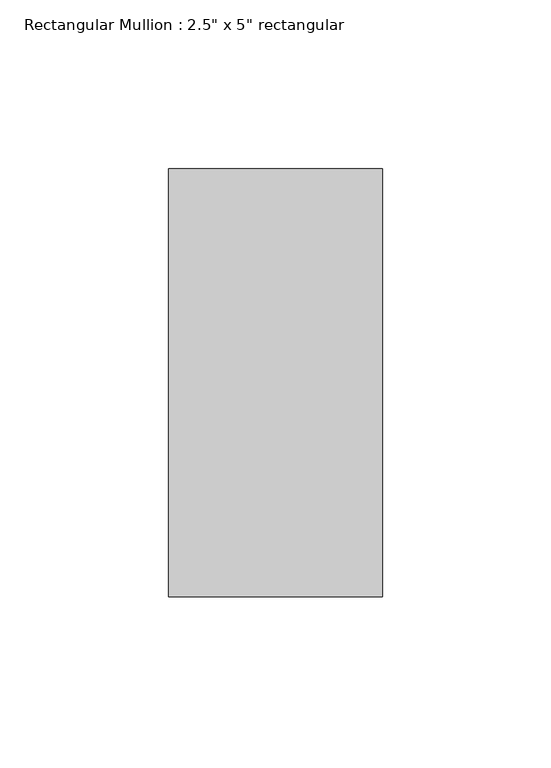
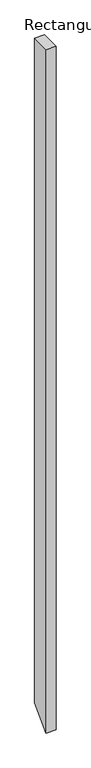
"""IFC4 building model written with IfcOpenShell, lengths in millimetres: member geometry."""

from ifc_helpers import new_model, si_unit, frame, origin, place, context, project, spatial, polyline, outline, extrude, source, transform, mapped, element, save


def member_cf286210(model_context):
    return source(origin(), model_context, "Body", "SweptSolid", [
        extrude(outline(polyline([(-63.5, 0.0), (63.5, 0.0), (63.5, -4482.350494), (-63.5, -4609.350494), (-63.5, 0.0)])), frame((-63.5, 0.0, 0.0), z_axis=(1.0, 0.0, 0.0), x_axis=(0.0, 1.0, 0.0)), (0.0, 0.0, 1.0), 63.5),
    ])


if __name__ == "__main__":
    model = new_model("IFC4")
    model_context = context("Model", 3, world=origin())
    ifc_project = project(units=[si_unit("LENGTHUNIT", "METRE", prefix="MILLI")], contexts=[model_context])
    site = spatial("IfcSite", under=ifc_project)
    building = spatial("IfcBuilding", under=site)
    placement = place(None, origin())
    member_shape = member_cf286210(model_context)
    element("IfcMember", 1, ObjectType="Rectangular Mullion : 2.5\" x 5\" rectangular", at=placement, inside=building, context=model_context, shape_type="MappedRepresentation", body=[
        mapped(member_shape, transform((0.0, 0.0, 0.0), x_axis=(1.0, 0.0, 0.0), y_axis=(0.0, 1.0, 0.0), z_axis=(0.0, 0.0, 1.0))),
    ])
    save(model, "model.ifc")

# Revit data of these elements
# Type "Rectangular Mullion : 2.5\" x 5\" rectangular"
#   built-in parameter 1007304 = 0.416667 (stored number, unit not read)
#   built-in parameter 1007301 = 0.104167 (stored number, unit not read)
#   built-in parameter 1007300 = 0.104167 (stored number, unit not read)
# Element 1 (IfcMember, "Rectangular Mullion : 2.5\" x 5\" rectangular")
#   Materials on its faces: "Aluminum"
# Materials
#   "Aluminum": class "Metal", colour RGB 247 247 247, transparency 0, Description = "Aluminum 6061", Cost = 0
